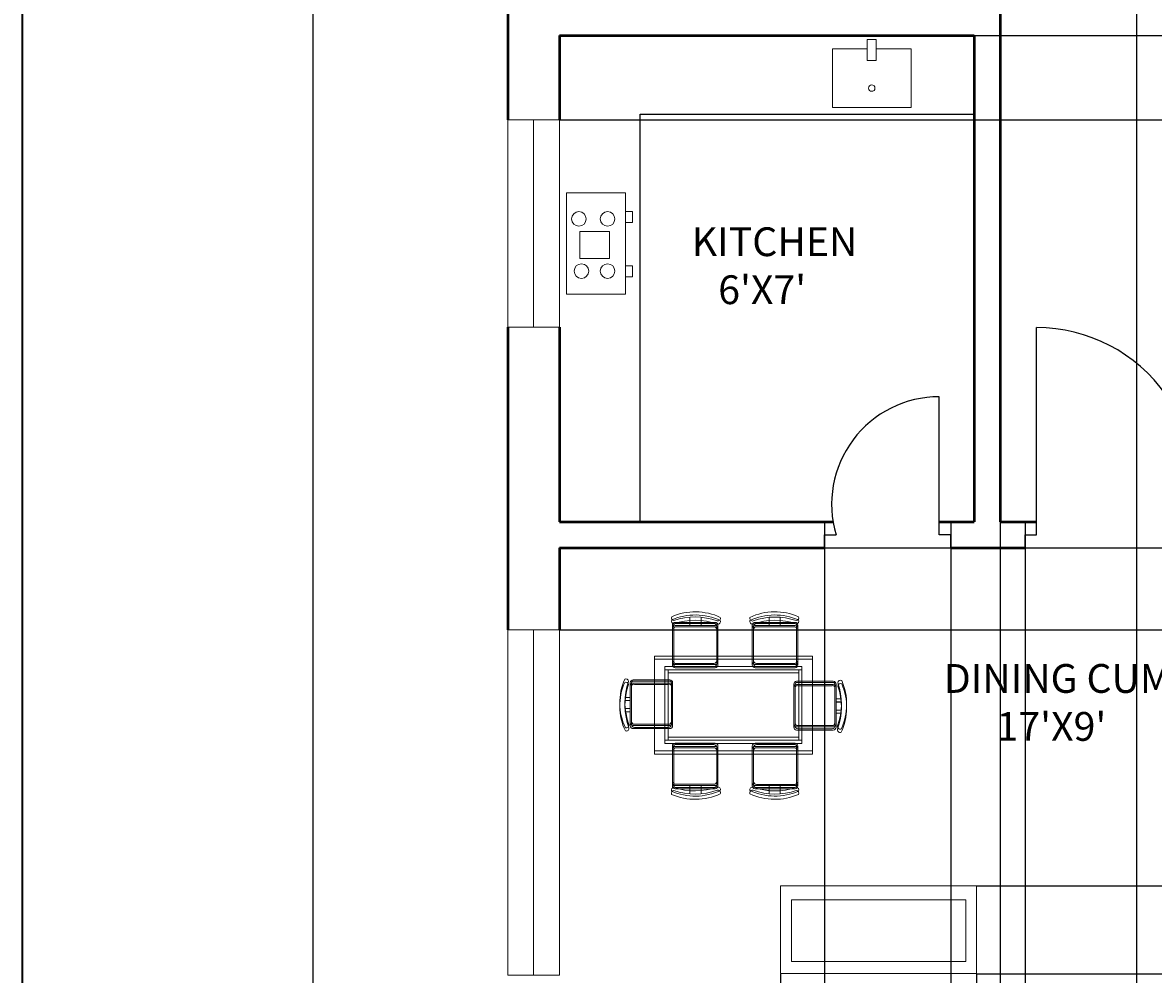
# Model space of a CAD drawing. Units: inches. Extents: x 2310 to 2937, y 1113 to 2410.
# Tile 17 of 23: x 2310 to 2507, y 2132 to 2297. Entities that reach past the tile are written whole.
import ezdxf

# ---------------------------------------------------------------- set-up
doc = ezdxf.new("R2010")
doc.units = ezdxf.units.IN
for name, color, linetype, lineweight in [('A-ANNO-DIMS', 2, 'Continuous', 18), ('A-ANNO-TTLB', 7, 'Continuous', 35), ('A-AREA-IDEN', 7, 'Continuous', 18), ('A-DOOR', 31, 'Continuous', 25), ('A-EQPM', 8, 'Continuous', 18), ('A-FLOR-CASE', 7, 'Continuous', 25), ('A-FLOR-FIXT', 9, 'Continuous', 18), ('A-FURN', 8, 'Continuous', 18), ('A-GLAZ', 191, 'Continuous', 20), ('A-WALL', 7, 'Continuous', 50)]:
    doc.layers.add(name, color=color, linetype=linetype, lineweight=lineweight)
doc.styles.get("Standard").update_dxf_attribs({"font": 'arial.ttf'})
doc.dimstyles.get("Standard").update_dxf_attribs({"dimtxt": 0.18, "dimasz": 0.18, "dimexe": 0.18, "dimexo": 0.0625, "dimgap": 0.09, "dimtad": 0, "dimtih": 1, "dimtoh": 1, "dimdec": 4, "dimzin": 0, "dimdsep": 46, "dimtxsty": 'Standard', "dimcen": 0.09, "dimadec": 0, "dimazin": 0, "dimtfac": 1, "dimtdec": 4, "dimtofl": 0, "dimtmove": 0, "dimatfit": 3, "dimfxl": 1, "dimtolj": 1, "dimtzin": 0, "dimarcsym": 0})

# ---------------------------------------------------------------- blocks, each defined once
blk = doc.blocks.new('SINK-KITCHEN')
blk.add_lwpolyline([(6.01, 11.79), (7.56, 11.79), (7.56, 8.11), (6.01, 8.11)], close=True)
blk.add_lwpolyline([(7.56, 10.17), (13.64, 10.17), (13.64, 0), (0, 0), (0, 10.17), (6.01, 10.17)])
blk.add_circle((6.79, 3.34), 0.556)
blk = doc.blocks.new('RANGE-4-BURNER')
for points in [[(1.2, 17.61), (1.2, 17.61), (1.2, 17.61), (1.2, 17.61)], [(1.2, 17.61), (11.5, 17.61), (11.5, 0), (1.2, 0)], [(1.2, 14.58), (0, 14.58), (0, 12.67), (1.2, 12.67)], [(4.01, 11.43), (9.13, 11.43), (9.13, 6.73), (4.01, 6.73)], [(1.2, 5.14), (0, 5.14), (0, 3.24), (1.2, 3.24)]]:
    blk.add_lwpolyline(points, close=True)
for centre in [(4.34, 13.6), (8.87, 13.6), (4.34, 4.53), (9.32, 4.53)]:
    blk.add_circle(centre, 1.27)
blk = doc.blocks.new('WIN-60IN')
for p, q in [((4.5, 60), (0, 60)), ((0, 60), (9, 60)), ((0, 60), (0, 0)), ((4.5, 0), (4.5, 60)), ((9, 60), (9, 0)), ((0, 0), (9, 0)), ((9, 0), (4.5, 0))]:
    blk.add_line(p, q)
blk = doc.blocks.new('DINING-TABLE')
for points in [[(0, 17.02), (27.45, 17.02), (27.45, 0.55), (0, 0.55)], [(0, 17.02), (27.45, 17.02), (27.45, 0.55), (0, 0.55)], [(0, 16.47), (27.45, 16.47), (27.45, 0), (0, 0)], [(0, 16.47), (27.45, 16.47), (27.45, 0), (0, 0)], [(1.83, 15.19), (25.62, 15.19), (25.62, 2.38), (1.83, 2.38)], [(1.83, 15.19), (25.62, 15.19), (25.62, 2.38), (1.83, 2.38)], [(1.83, 14.64), (25.62, 14.64), (25.62, 1.83), (1.83, 1.83)], [(1.83, 14.64), (25.62, 14.64), (25.62, 1.83), (1.83, 1.83)], [(2.38, 14.64), (25.07, 14.64), (25.07, 2.93), (2.38, 2.93)], [(2.38, 14.64), (25.07, 14.64), (25.07, 2.93), (2.38, 2.93)], [(2.38, 14.09), (25.07, 14.09), (25.07, 2.38), (2.38, 2.38)], [(2.38, 14.09), (25.07, 14.09), (25.07, 2.38), (2.38, 2.38)]]:
    blk.add_lwpolyline(points, close=True)
blk = doc.blocks.new('CHAIR-DINING')
for points in [[(0.62, 8.14, -0.578392), (0.05, 8.77, -0.214524), (8.49, 8.88, -0.552014), (8.09, 8.2, 0.175809), (0.62, 8.14)], [(0.62, 8.14, -0.578392), (0.05, 8.77, -0.214524), (8.49, 8.88, -0.552014), (8.09, 8.2, 0.175809), (0.62, 8.14)], [(0.62, 7.6, -0.578392), (0.05, 8.22, -0.214524), (8.49, 8.33, -0.552014), (8.09, 7.65, 0.175809), (0.62, 7.6)], [(0.62, 7.6, -0.578392), (0.05, 8.22, -0.214524), (8.49, 8.33, -0.552014), (8.09, 7.65, 0.175809), (0.62, 7.6)], [(7.88, 7.9, -0.414214), (8.36, 7.42), (8.36, 1.03, -0.414214), (7.88, 0.55), (0.94, 0.55, -0.414214), (0.45, 1.03), (0.45, 7.42, -0.414214), (0.94, 7.9), (7.88, 7.9)], [(7.88, 7.9, -0.414214), (8.36, 7.42), (8.36, 1.03, -0.414214), (7.88, 0.55), (0.94, 0.55, -0.414214), (0.45, 1.03), (0.45, 7.42, -0.414214), (0.94, 7.9), (7.88, 7.9)], [(3.37, 7.9), (3.37, 8.78, 0.064759)], [(3.37, 7.9), (3.37, 8.78, 0.064759)], [(3.37, 7.35), (3.37, 8.23, 0.064759)], [(3.37, 7.35), (3.37, 8.23, 0.064759)], [(7.88, 7.35, -0.414214), (8.36, 6.87), (8.36, 0.49, -0.414214), (7.88, 0), (0.94, 0, -0.414214), (0.45, 0.49), (0.45, 6.87, -0.414214), (0.94, 7.35), (7.88, 7.35)], [(7.88, 7.35, -0.414214), (8.36, 6.87), (8.36, 0.49, -0.414214), (7.88, 0), (0.94, 0, -0.414214), (0.45, 0.49), (0.45, 6.87, -0.414214), (0.94, 7.35), (7.88, 7.35)]]:
    blk.add_lwpolyline(points, format="xyb")
for points in [[(5.32, 8.8), (5.32, 7.9)], [(5.32, 8.79), (5.32, 7.9)], [(5.32, 8.25), (5.32, 7.35)], [(5.32, 8.25), (5.32, 7.35)]]:
    blk.add_lwpolyline(points)
for points in [[(7.87, 7.68), (1.16, 7.68, 0.414214), (0.67, 7.2), (0.67, 1.25, 0.414214), (1.16, 0.77), (7.87, 0.77, 0.512069), (8.14, 1.25), (8.14, 7.2, 0.512069)], [(7.87, 7.68), (1.16, 7.68, 0.414214), (0.67, 7.2), (0.67, 1.25, 0.414214), (1.16, 0.77), (7.87, 0.77, 0.512069), (8.14, 1.25), (8.14, 7.2, 0.512069)], [(7.87, 7.13), (1.16, 7.13, 0.414214), (0.67, 6.65), (0.67, 0.7, 0.414214), (1.16, 0.22), (7.87, 0.22, 0.512069), (8.14, 0.7), (8.14, 6.65, 0.512069)], [(7.87, 7.13), (1.16, 7.13, 0.414214), (0.67, 6.65), (0.67, 0.7, 0.414214), (1.16, 0.22), (7.87, 0.22, 0.512069), (8.14, 0.7), (8.14, 6.65, 0.512069)]]:
    blk.add_lwpolyline(points, format="xyb", close=True)
blk = doc.blocks.new('CHAIR-DINING-2')
for points in [[(7.63, 2.7), (0.69, 2.7, -0.414214), (0.2, 3.18), (0.2, 9.57, -0.414214), (0.69, 10.05), (7.63, 10.05, -0.414214), (8.11, 9.57), (8.11, 3.18, -0.414214), (7.63, 2.7)], [(7.63, 2.7), (0.69, 2.7, -0.414214), (0.2, 3.18), (0.2, 9.57, -0.414214), (0.69, 10.05), (7.63, 10.05, -0.414214), (8.11, 9.57), (8.11, 3.18, -0.414214), (7.63, 2.7)], [(7.63, 2.15), (0.69, 2.15, -0.414214), (0.2, 2.64), (0.2, 9.02, -0.414214), (0.69, 9.5), (7.63, 9.5, -0.414214), (8.11, 9.02), (8.11, 2.64, -0.414214), (7.63, 2.15)], [(7.63, 2.15), (0.69, 2.15, -0.414214), (0.2, 2.64), (0.2, 9.02, -0.414214), (0.69, 9.5), (7.63, 9.5, -0.414214), (8.11, 9.02), (8.11, 2.64, -0.414214), (7.63, 2.15)], [(7.95, 2.46, -0.578392), (8.51, 1.83, -0.214524), (0.07, 1.72, -0.552014), (0.47, 2.4, 0.175809), (7.95, 2.46)], [(7.95, 2.46, -0.578392), (8.51, 1.83, -0.214524), (0.07, 1.72, -0.552014), (0.47, 2.4, 0.175809), (7.95, 2.46)], [(5.19, 2.7), (5.19, 1.82, 0.064759)], [(5.19, 2.7), (5.19, 1.82, 0.064759)], [(5.19, 2.15), (5.19, 1.27, 0.064759)], [(5.19, 2.15), (5.19, 1.27, 0.064759)], [(7.95, 1.91, -0.578392), (8.51, 1.28, -0.214524), (0.07, 1.17, -0.552014), (0.47, 1.85, 0.175809), (7.95, 1.91)], [(7.95, 1.91, -0.578392), (8.51, 1.28, -0.214524), (0.07, 1.17, -0.552014), (0.47, 1.85, 0.175809), (7.95, 1.91)]]:
    blk.add_lwpolyline(points, format="xyb")
for points in [[(0.69, 2.92), (7.41, 2.92, 0.414214), (7.9, 3.4), (7.9, 9.35, 0.414214), (7.41, 9.83), (0.69, 9.83, 0.512069), (0.42, 9.35), (0.42, 3.4, 0.512069)], [(0.69, 2.92), (7.41, 2.92, 0.414214), (7.9, 3.4), (7.9, 9.35, 0.414214), (7.41, 9.83), (0.69, 9.83, 0.512069), (0.42, 9.35), (0.42, 3.4, 0.512069)], [(0.69, 2.37), (7.41, 2.37, 0.414214), (7.9, 2.85), (7.9, 8.8, 0.414214), (7.41, 9.28), (0.69, 9.28, 0.512069), (0.42, 8.8), (0.42, 2.85, 0.512069)], [(0.69, 2.37), (7.41, 2.37, 0.414214), (7.9, 2.85), (7.9, 8.8, 0.414214), (7.41, 9.28), (0.69, 9.28, 0.512069), (0.42, 8.8), (0.42, 2.85, 0.512069)]]:
    blk.add_lwpolyline(points, format="xyb", close=True)
for points in [[(3.25, 1.81), (3.25, 2.7)], [(3.25, 1.81), (3.25, 2.7)], [(3.25, 1.26), (3.25, 2.15)], [(3.25, 1.26), (3.25, 2.15)]]:
    blk.add_lwpolyline(points)
blk = doc.blocks.new('*D40')
at = {"layer": 'A-ANNO-DIMS', "color": 0, "lineweight": -2, "transparency": 16777216}
for p, q in [((2394.42, 2356.51), (2360.46, 2356.51)), ((2360.64, 2356.33), (2360.64, 2046.7)), ((2360.64, 1736.69), (2360.64, 2046.33)), ((2394.42, 1736.51), (2360.46, 1736.51))]:
    blk.add_line(p, q, dxfattribs=at)
at = {"layer": 'A-ANNO-DIMS', "color": 0, "transparency": 16777216}
for points in [[(2360.61, 2356.33), (2360.67, 2356.33), (2360.64, 2356.51)], [(2360.61, 1736.69), (2360.67, 1736.69), (2360.64, 1736.51)]]:
    blk.add_solid(points, dxfattribs=at)
at = {"layer": 'Defpoints', "color": 0, "transparency": 16777216}
for p in [(2360.64, 2356.51), (2394.49, 2356.51), (2394.49, 1736.51)]:
    blk.add_point(p, dxfattribs=at)
at = {"layer": 'A-ANNO-DIMS', "color": 0, "transparency": 16777216, "insert": (2360.64, 2046.51), "char_height": 0.18, "attachment_point": 5}
blk.add_mtext('\\A1;620', dxfattribs=at)
blk = doc.blocks.new('*D41')
at = {"layer": 'A-ANNO-DIMS', "color": 0, "lineweight": -2, "transparency": 16777216}
for p, q in [((2479.99, 2347.45), (2479.99, 1649.5)), ((2503.66, 2347.45), (2503.66, 1649.5)), ((2480.17, 1649.68), (2491.36, 1649.68)), ((2503.48, 1649.68), (2492.29, 1649.68))]:
    blk.add_line(p, q, dxfattribs=at)
at = {"layer": 'A-ANNO-DIMS', "color": 0, "transparency": 16777216}
for points in [[(2480.17, 1649.71), (2480.17, 1649.65), (2479.99, 1649.68)], [(2503.48, 1649.71), (2503.48, 1649.65), (2503.66, 1649.68)]]:
    blk.add_solid(points, dxfattribs=at)
at = {"layer": 'Defpoints', "color": 0, "transparency": 16777216}
for p in [(2479.99, 2347.51), (2503.66, 2347.51), (2503.66, 1649.68)]:
    blk.add_point(p, dxfattribs=at)
at = {"layer": 'A-ANNO-DIMS', "color": 0, "transparency": 16777216, "insert": (2491.82, 1649.68), "char_height": 0.18, "attachment_point": 5}
blk.add_mtext('\\A1;23.676', dxfattribs=at)
blk = doc.blocks.new('*D53')
at = {"layer": 'A-ANNO-DIMS', "color": 0, "lineweight": -2, "transparency": 16777216}
for p, q in [((2403.55, 2295.01), (2858.02, 2295.01)), ((2857.84, 2294.83), (2857.84, 2287.87)), ((2857.84, 2280.55), (2857.84, 2287.51)), ((2403.55, 2280.37), (2858.02, 2280.37))]:
    blk.add_line(p, q, dxfattribs=at)
at = {"layer": 'A-ANNO-DIMS', "color": 0, "transparency": 16777216}
for points in [[(2857.81, 2294.83), (2857.87, 2294.83), (2857.84, 2295.01)], [(2857.81, 2280.55), (2857.87, 2280.55), (2857.84, 2280.37)]]:
    blk.add_solid(points, dxfattribs=at)
at = {"layer": 'Defpoints', "color": 0, "transparency": 16777216}
for p in [(2403.49, 2295.01), (2403.49, 2280.37), (2857.84, 2280.37)]:
    blk.add_point(p, dxfattribs=at)
at = {"layer": 'A-ANNO-DIMS', "color": 0, "transparency": 16777216, "insert": (2857.84, 2287.69), "char_height": 0.18, "attachment_point": 5}
blk.add_mtext('\\A1;14.644', dxfattribs=at)
blk = doc.blocks.new('*D54')
at = {"layer": 'A-ANNO-DIMS', "color": 0, "lineweight": -2, "transparency": 16777216}
for p, q in [((2403.55, 2206.01), (2858.02, 2206.01)), ((2857.84, 2205.83), (2857.84, 2199.07)), ((2857.84, 2191.94), (2857.84, 2198.7)), ((2403.55, 2191.76), (2858.02, 2191.76))]:
    blk.add_line(p, q, dxfattribs=at)
at = {"layer": 'A-ANNO-DIMS', "color": 0, "transparency": 16777216}
for points in [[(2857.81, 2205.83), (2857.87, 2205.83), (2857.84, 2206.01)], [(2857.81, 2191.94), (2857.87, 2191.94), (2857.84, 2191.76)]]:
    blk.add_solid(points, dxfattribs=at)
at = {"layer": 'Defpoints', "color": 0, "transparency": 16777216}
for p in [(2403.49, 2206.01), (2403.49, 2191.76), (2857.84, 2191.76)]:
    blk.add_point(p, dxfattribs=at)
at = {"layer": 'A-ANNO-DIMS', "color": 0, "transparency": 16777216, "insert": (2857.84, 2198.89), "char_height": 0.18, "attachment_point": 5}
blk.add_mtext('\\A1;14.255', dxfattribs=at)
blk = doc.blocks.new('*D60')
at = {"layer": 'A-ANNO-DIMS', "color": 0, "lineweight": -2, "transparency": 16777216}
for p, q in [((2449.5, 2205.95), (2449.5, 1649.5)), ((2471.44, 2205.95), (2471.44, 1649.5)), ((2449.68, 1649.68), (2460.01, 1649.68)), ((2471.26, 1649.68), (2460.94, 1649.68))]:
    blk.add_line(p, q, dxfattribs=at)
at = {"layer": 'A-ANNO-DIMS', "color": 0, "transparency": 16777216}
for points in [[(2449.68, 1649.71), (2449.68, 1649.65), (2449.5, 1649.68)], [(2471.26, 1649.71), (2471.26, 1649.65), (2471.44, 1649.68)]]:
    blk.add_solid(points, dxfattribs=at)
at = {"layer": 'Defpoints', "color": 0, "transparency": 16777216}
for p in [(2449.5, 2206.01), (2471.44, 2206.01), (2471.44, 1649.68)]:
    blk.add_point(p, dxfattribs=at)
at = {"layer": 'A-ANNO-DIMS', "color": 0, "transparency": 16777216, "insert": (2460.47, 1649.68), "char_height": 0.18, "attachment_point": 5}
blk.add_mtext('\\A1;21.936', dxfattribs=at)
blk = doc.blocks.new('*D61')
at = {"layer": 'A-ANNO-DIMS', "color": 0, "lineweight": -2, "transparency": 16777216}
for p, q in [((2484.33, 2205.95), (2484.33, 1649.5)), ((2514.27, 2205.95), (2514.27, 1649.5)), ((2484.51, 1649.68), (2498.9, 1649.68)), ((2514.09, 1649.68), (2499.69, 1649.68))]:
    blk.add_line(p, q, dxfattribs=at)
at = {"layer": 'A-ANNO-DIMS', "color": 0, "transparency": 16777216}
for points in [[(2484.51, 1649.71), (2484.51, 1649.65), (2484.33, 1649.68)], [(2514.09, 1649.71), (2514.09, 1649.65), (2514.27, 1649.68)]]:
    blk.add_solid(points, dxfattribs=at)
at = {"layer": 'Defpoints', "color": 0, "transparency": 16777216}
for p in [(2484.33, 2206.01), (2514.27, 2206.01), (2514.27, 1649.68)]:
    blk.add_point(p, dxfattribs=at)
at = {"layer": 'A-ANNO-DIMS', "color": 0, "transparency": 16777216, "insert": (2499.3, 1649.68), "char_height": 0.18, "attachment_point": 5}
blk.add_mtext('\\A1;29.94', dxfattribs=at)
blk = doc.blocks.new('*D69')
at = {"layer": 'A-ANNO-DIMS', "color": 0, "lineweight": -2, "transparency": 16777216}
for p, q in [((2441.86, 2131.96), (2441.86, 1649.5)), ((2475.89, 2131.96), (2475.89, 1649.5)), ((2442.04, 1649.68), (2458.48, 1649.68)), ((2475.71, 1649.68), (2459.27, 1649.68))]:
    blk.add_line(p, q, dxfattribs=at)
at = {"layer": 'A-ANNO-DIMS', "color": 0, "transparency": 16777216}
for points in [[(2442.04, 1649.71), (2442.04, 1649.65), (2441.86, 1649.68)], [(2475.71, 1649.71), (2475.71, 1649.65), (2475.89, 1649.68)]]:
    blk.add_solid(points, dxfattribs=at)
at = {"layer": 'Defpoints', "color": 0, "transparency": 16777216}
for p in [(2441.86, 2132.02), (2475.89, 2132.02), (2475.89, 1649.68)]:
    blk.add_point(p, dxfattribs=at)
at = {"layer": 'A-ANNO-DIMS', "color": 0, "transparency": 16777216, "insert": (2458.88, 1649.68), "char_height": 0.18, "attachment_point": 5}
blk.add_mtext('\\A1;34.03', dxfattribs=at)
blk = doc.blocks.new('*D70')
at = {"layer": 'A-ANNO-DIMS', "color": 0, "lineweight": -2, "transparency": 16777216}
for p, q in [((2475.96, 2147.28), (2858.02, 2147.28)), ((2857.84, 2147.1), (2857.84, 2139.83)), ((2857.84, 2132.2), (2857.84, 2139.47)), ((2475.96, 2132.02), (2858.02, 2132.02))]:
    blk.add_line(p, q, dxfattribs=at)
at = {"layer": 'A-ANNO-DIMS', "color": 0, "transparency": 16777216}
for points in [[(2857.81, 2147.1), (2857.87, 2147.1), (2857.84, 2147.28)], [(2857.81, 2132.2), (2857.87, 2132.2), (2857.84, 2132.02)]]:
    blk.add_solid(points, dxfattribs=at)
at = {"layer": 'Defpoints', "color": 0, "transparency": 16777216}
for p in [(2475.89, 2147.28), (2857.84, 2147.28), (2475.89, 2132.02)]:
    blk.add_point(p, dxfattribs=at)
at = {"layer": 'A-ANNO-DIMS', "color": 0, "transparency": 16777216, "insert": (2857.84, 2139.65), "char_height": 0.18, "attachment_point": 5}
blk.add_mtext('\\A1;15.257', dxfattribs=at)

msp = doc.modelspace()

# ---------------------------------------------------------------- linework, layer by layer
at = {"layer": 'A-ANNO-TTLB'}
msp.add_lwpolyline([(2310.2498, 2409.8427), (2937.0534, 2409.8427), (2937.0534, 1616.036), (2310.2498, 1616.036)], close=True, dxfattribs=at)
at = {"layer": 'A-DOOR'}
for p, q in [((2486.3278, 2208.2639), (2486.3278, 2244.2639)), ((2469.4388, 2208.2639), (2469.4388, 2232.2639)), ((2449.5024, 2210.5139), (2449.5024, 2206.0139)), ((2471.4388, 2210.5139), (2471.4388, 2206.0139)), ((2484.3278, 2210.5139), (2484.3278, 2206.0139)), ((2449.5024, 2206.0139), (2449.5024, 2208.2639)), ((2449.5024, 2208.2639), (2451.5024, 2208.2639)), ((2471.4388, 2208.2639), (2469.4388, 2208.2639)), ((2471.4388, 2206.0139), (2471.4388, 2208.2639)), ((2484.3278, 2206.0139), (2484.3278, 2208.2639)), ((2484.3278, 2208.2639), (2486.3278, 2208.2639))]:
    msp.add_line(p, q, dxfattribs=at)
for centre, radius, start, end in [((2486.3278, 2216.7342), 27.5298, 340.442065, 90), ((2469.4388, 2213.5616), 18.7023, 90, 196.455037)]:
    msp.add_arc(centre, radius, start, end, dxfattribs=at)
at = {"layer": 'A-FLOR-CASE'}
for p, q in [((2417.517, 2210.5139), (2417.517, 2281.346)), ((2417.517, 2281.346), (2471.5691, 2281.346)), ((2471.5691, 2281.346), (2475.4859, 2281.346))]:
    msp.add_line(p, q, dxfattribs=at)
at = {"layer": 'A-FURN'}
for points in [[(2423.3618, 2193.3629, -0.17580919), (2430.8373, 2193.3063, 0.57839206), (2431.4036, 2193.929, 0.21452438), (2422.9654, 2194.0423, 0.55201397), (2423.3618, 2193.3629, -0.06507904)], [(2423.3618, 2193.3626, -0.17580919), (2430.8373, 2193.306, 0.57839206), (2431.4036, 2193.9287, 0.21452438), (2422.9654, 2194.042, 0.55201397), (2423.3618, 2193.3626, -0.06507904)], [(2423.3618, 2192.814, -0.17580919), (2430.8373, 2192.7574, 0.57839206), (2431.4036, 2193.3801, 0.21452438), (2422.9654, 2193.4933, 0.55201397), (2423.3618, 2192.814, -0.06507904)], [(2423.3618, 2192.8137, -0.17580919), (2430.8373, 2192.7571, 0.57839206), (2431.4036, 2193.3798, 0.21452438), (2422.9654, 2193.493, 0.55201397), (2423.3618, 2192.8137, -0.06507904)], [(2428.0825, 2193.0629), (2428.0825, 2193.9406, -0.06475861)], [(2428.0825, 2193.0626), (2428.0825, 2193.9403, -0.06475861)], [(2430.5201, 2193.0629), (2423.5802, 2193.0629, 0.41421356), (2423.0946, 2192.5774), (2423.0946, 2186.1962, 0.41421356), (2423.5802, 2185.7107), (2430.5201, 2185.7107, 0.41421356), (2431.0056, 2186.1962), (2431.0056, 2192.5774, 0.41421356), (2430.5201, 2193.0629)], [(2430.5201, 2192.514), (2423.5802, 2192.514, 0.41421356), (2423.0946, 2192.0285), (2423.0946, 2185.6473, 0.41421356), (2423.5802, 2185.1618), (2430.5201, 2185.1618, 0.41421356), (2431.0056, 2185.6473), (2431.0056, 2192.0285, 0.41421356), (2430.5201, 2192.514)], [(2430.5201, 2193.0626), (2423.5802, 2193.0626, 0.41421356), (2423.0947, 2192.5771), (2423.0947, 2186.1959, 0.41421356), (2423.5802, 2185.7104), (2430.5201, 2185.7104, 0.41421356), (2431.0056, 2186.1959), (2431.0056, 2192.5771, 0.41421356), (2430.5201, 2193.0626)], [(2430.5201, 2192.5137), (2423.5802, 2192.5137, 0.41421356), (2423.0947, 2192.0282), (2423.0947, 2185.647, 0.41421356), (2423.5802, 2185.1615), (2430.5201, 2185.1615, 0.41421356), (2431.0056, 2185.647), (2431.0056, 2192.0282, 0.41421356), (2430.5201, 2192.5137)], [(2428.0825, 2192.514), (2428.0825, 2193.3917, -0.06475861)], [(2428.0825, 2192.5137), (2428.0825, 2193.3914, -0.06475861)], [(2415.5411, 2175.3109, -0.57839206), (2414.9184, 2174.7446, -0.21452438), (2414.8051, 2183.1827, -0.55201397), (2415.4845, 2182.7863, 0.17580937), (2415.5411, 2175.3109)], [(2415.5411, 2175.3106, -0.57839206), (2414.9184, 2174.7443, -0.21452438), (2414.8052, 2183.1825, -0.55201397), (2415.4845, 2182.786, 0.17580937), (2415.5411, 2175.3106)], [(2415.5411, 2174.762, -0.57839206), (2414.9184, 2174.1956, -0.21452438), (2414.8051, 2182.6338, -0.55201397), (2415.4845, 2182.2374, 0.17580937), (2415.5411, 2174.762)], [(2415.5411, 2174.7617, -0.57839206), (2414.9184, 2174.1954, -0.21452438), (2414.8052, 2182.6335, -0.55201397), (2415.4845, 2182.2371, 0.17580937), (2415.5411, 2174.7617)], [(2415.7845, 2182.568, -0.41421356), (2416.27, 2183.0535), (2422.6512, 2183.0535, -0.41421356), (2423.1367, 2182.568), (2423.1367, 2175.628, -0.41421356), (2422.6512, 2175.1425), (2416.27, 2175.1425, -0.41421356), (2415.7845, 2175.628), (2415.7845, 2182.568)], [(2415.7845, 2182.5677, -0.41421356), (2416.27, 2183.0532), (2422.6512, 2183.0532, -0.41421356), (2423.1367, 2182.5677), (2423.1367, 2175.6277, -0.41421356), (2422.6512, 2175.1422), (2416.27, 2175.1422, -0.41421356), (2415.7845, 2175.6277), (2415.7845, 2182.5677)], [(2415.7845, 2182.0191, -0.41421356), (2416.27, 2182.5046), (2422.6512, 2182.5046, -0.41421356), (2423.1367, 2182.0191), (2423.1367, 2175.0791, -0.41421356), (2422.6512, 2174.5936), (2416.27, 2174.5936, -0.41421356), (2415.7845, 2175.0791), (2415.7845, 2182.0191)], [(2415.7845, 2182.0188, -0.41421356), (2416.27, 2182.5043), (2422.6512, 2182.5043, -0.41421356), (2423.1367, 2182.0188), (2423.1367, 2175.0788, -0.41421356), (2422.6512, 2174.5933), (2416.27, 2174.5933, -0.41421356), (2415.7845, 2175.0788), (2415.7845, 2182.0188)], [(2451.522, 2182.3303, 0.41421356), (2451.0364, 2182.8158), (2444.6553, 2182.8158, 0.41421356), (2444.1698, 2182.3303), (2444.1698, 2175.3904, 0.41421356), (2444.6553, 2174.9048), (2451.0364, 2174.9048, 0.41421356), (2451.522, 2175.3904), (2451.522, 2182.3303)], [(2451.522, 2182.33, 0.41421356), (2451.0364, 2182.8155), (2444.6553, 2182.8155, 0.41421356), (2444.1698, 2182.33), (2444.1698, 2175.3901, 0.41421356), (2444.6553, 2174.9045), (2451.0364, 2174.9045, 0.41421356), (2451.522, 2175.3901), (2451.522, 2182.33)], [(2451.522, 2181.7814, 0.41421356), (2451.0364, 2182.2669), (2444.6553, 2182.2669, 0.41421356), (2444.1698, 2181.7814), (2444.1698, 2174.8414, 0.41421356), (2444.6553, 2174.3559), (2451.0364, 2174.3559, 0.41421356), (2451.522, 2174.8414), (2451.522, 2181.7814)], [(2451.522, 2181.7811, 0.41421356), (2451.0364, 2182.2666), (2444.6553, 2182.2666, 0.41421356), (2444.1698, 2181.7811), (2444.1698, 2174.8411, 0.41421356), (2444.6553, 2174.3556), (2451.0364, 2174.3556, 0.41421356), (2451.522, 2174.8411), (2451.522, 2181.7811)], [(2451.822, 2182.5486, -0.17580919), (2451.7654, 2175.0732, 0.57839206), (2452.3881, 2174.5069, 0.21452438), (2452.5013, 2182.9451, 0.55201397), (2451.822, 2182.5486, -0.06507904)], [(2451.822, 2182.5483, -0.17580919), (2451.7654, 2175.0729, 0.57839206), (2452.3881, 2174.5066, 0.21452438), (2452.5013, 2182.9448, 0.55201397), (2451.822, 2182.5483, -0.06507904)], [(2451.822, 2181.9997, -0.17580919), (2451.7654, 2174.5243, 0.57839206), (2452.3881, 2173.958, 0.21452438), (2452.5013, 2182.3961, 0.55201397), (2451.822, 2181.9997, -0.06507904)], [(2451.822, 2181.9994, -0.17580919), (2451.7654, 2174.524, 0.57839206), (2452.3881, 2173.9577, 0.21452438), (2452.5013, 2182.3959, 0.55201397), (2451.822, 2181.9994, -0.06507904)], [(2415.7845, 2178.0657), (2414.9068, 2178.0657, 0.06475861)], [(2415.7845, 2178.0654), (2414.9068, 2178.0654, 0.06475861)], [(2451.522, 2177.828), (2452.3996, 2177.828, -0.06475861)], [(2451.522, 2177.8277), (2452.3997, 2177.8277, -0.06475861)], [(2415.7845, 2177.5168), (2414.9068, 2177.5168, 0.06475861)], [(2415.7845, 2177.5165), (2414.9068, 2177.5165, 0.06475861)], [(2451.522, 2177.2791), (2452.3996, 2177.2791, -0.06475861)], [(2451.522, 2177.2788), (2452.3997, 2177.2788, -0.06475861)], [(2444.3877, 2164.6971, 0.41421356), (2444.8732, 2165.1827), (2444.8732, 2171.5638, 0.41421356), (2444.3877, 2172.0493), (2437.4478, 2172.0493, 0.41421356), (2436.9622, 2171.5638), (2436.9622, 2165.1827, 0.41421356), (2437.4478, 2164.6971), (2444.3877, 2164.6971)], [(2444.3877, 2164.6969, 0.41421356), (2444.8732, 2165.1824), (2444.8732, 2171.5635, 0.41421356), (2444.3877, 2172.0491), (2437.4478, 2172.0491, 0.41421356), (2436.9623, 2171.5635), (2436.9623, 2165.1824, 0.41421356), (2437.4478, 2164.6969), (2444.3877, 2164.6969)], [(2444.3877, 2164.1482, 0.41421356), (2444.8732, 2164.6338), (2444.8732, 2171.0149, 0.41421356), (2444.3877, 2171.5004), (2437.4478, 2171.5004, 0.41421356), (2436.9622, 2171.0149), (2436.9622, 2164.6338, 0.41421356), (2437.4478, 2164.1482), (2444.3877, 2164.1482)], [(2444.3877, 2164.1479, 0.41421356), (2444.8732, 2164.6335), (2444.8732, 2171.0146, 0.41421356), (2444.3877, 2171.5001), (2437.4478, 2171.5001, 0.41421356), (2436.9623, 2171.0146), (2436.9623, 2164.6335, 0.41421356), (2437.4478, 2164.1479), (2444.3877, 2164.1479)], [(2444.606, 2164.3971, -0.17580928), (2437.1306, 2164.4537, 0.57839206), (2436.5643, 2163.831, 0.21452438), (2445.0025, 2163.7178, 0.55201397), (2444.6061, 2164.3971, -0.06507904)], [(2444.6061, 2164.3968, -0.17580928), (2437.1306, 2164.4534, 0.57839206), (2436.5643, 2163.8307, 0.21452438), (2445.0025, 2163.7175, 0.55201397), (2444.6061, 2164.3968, -0.06507904)], [(2439.8854, 2164.6971), (2439.8854, 2163.8195, -0.06475861)], [(2439.8854, 2164.6969), (2439.8854, 2163.8192, -0.06475861)], [(2439.8854, 2164.1482), (2439.8854, 2163.2705, -0.06475861)], [(2439.8854, 2164.1479), (2439.8854, 2163.2703, -0.06475861)], [(2444.606, 2163.8482, -0.17580928), (2437.1306, 2163.9048, 0.57839206), (2436.5643, 2163.2821, 0.21452438), (2445.0025, 2163.1689, 0.55201397), (2444.6061, 2163.8482, -0.06507904)], [(2444.6061, 2163.8479, -0.17580928), (2437.1306, 2163.9045, 0.57839206), (2436.5643, 2163.2818, 0.21452438), (2445.0025, 2163.1686, 0.55201397), (2444.6061, 2163.8479, -0.06507904)]]:
    msp.add_lwpolyline(points, format="xyb", dxfattribs=at)
for points in [[(2426.1399, 2193.9565), (2426.1399, 2193.0629)], [(2426.1399, 2193.9562), (2426.1399, 2193.0626)], [(2426.1399, 2193.4076), (2426.1399, 2192.514)], [(2426.1399, 2193.4073), (2426.1399, 2192.5137)], [(2414.8909, 2180.0083), (2415.7845, 2180.0083)], [(2414.8909, 2180.008), (2415.7845, 2180.008)], [(2452.4156, 2179.7706), (2451.522, 2179.7706)], [(2452.4156, 2179.7703), (2451.522, 2179.7703)], [(2414.8909, 2179.4594), (2415.7845, 2179.4594)], [(2414.8909, 2179.4591), (2415.7845, 2179.4591)], [(2452.4156, 2179.2217), (2451.522, 2179.2217)], [(2452.4156, 2179.2214), (2451.522, 2179.2214)], [(2441.828, 2163.8035), (2441.828, 2164.6971)], [(2441.828, 2163.8032), (2441.828, 2164.6969)], [(2441.828, 2163.2546), (2441.828, 2164.1482)], [(2441.828, 2163.2543), (2441.828, 2164.1479)]]:
    msp.add_lwpolyline(points, dxfattribs=at)
for points in [[(2423.5831, 2192.8442), (2430.3014, 2192.8442, -0.41421356), (2430.7869, 2192.3586), (2430.7869, 2186.415, -0.41421356), (2430.3014, 2185.9294), (2423.5831, 2185.9294, -0.51206948), (2423.3134, 2186.415), (2423.3134, 2192.3586, -0.51206948)], [(2423.5831, 2192.8439), (2430.3014, 2192.8439, -0.41421356), (2430.7869, 2192.3583), (2430.7869, 2186.4147, -0.41421356), (2430.3014, 2185.9291), (2423.5831, 2185.9291, -0.51206948), (2423.3134, 2186.4147), (2423.3134, 2192.3583, -0.51206948)], [(2423.5831, 2192.2952), (2430.3014, 2192.2952, -0.41421356), (2430.7869, 2191.8097), (2430.7869, 2185.866, -0.41421356), (2430.3014, 2185.3805), (2423.5831, 2185.3805, -0.51206948), (2423.3134, 2185.866), (2423.3134, 2191.8097, -0.51206948)], [(2423.5831, 2192.295), (2430.3014, 2192.295, -0.41421356), (2430.7869, 2191.8094), (2430.7869, 2185.8658, -0.41421356), (2430.3014, 2185.3802), (2423.5831, 2185.3802, -0.51206948), (2423.3134, 2185.8658), (2423.3134, 2191.8094, -0.51206948)], [(2416.0032, 2182.565), (2416.0032, 2175.8468, 0.41421356), (2416.4888, 2175.3612), (2422.4324, 2175.3612, 0.41421356), (2422.918, 2175.8468), (2422.918, 2182.565, 0.51206948), (2422.4324, 2182.8348), (2416.4888, 2182.8348, 0.51206948)], [(2416.0032, 2182.5647), (2416.0032, 2175.8465, 0.41421356), (2416.4888, 2175.3609), (2422.4325, 2175.3609, 0.41421356), (2422.918, 2175.8465), (2422.918, 2182.5647, 0.51206948), (2422.4325, 2182.8345), (2416.4888, 2182.8345, 0.51206948)], [(2416.0032, 2182.0161), (2416.0032, 2175.2978, 0.41421356), (2416.4888, 2174.8123), (2422.4324, 2174.8123, 0.41421356), (2422.918, 2175.2978), (2422.918, 2182.0161, 0.51206948), (2422.4324, 2182.2859), (2416.4888, 2182.2859, 0.51206948)], [(2416.0032, 2182.0158), (2416.0032, 2175.2976, 0.41421356), (2416.4888, 2174.812), (2422.4325, 2174.812, 0.41421356), (2422.918, 2175.2976), (2422.918, 2182.0158, 0.51206948), (2422.4325, 2182.2856), (2416.4888, 2182.2856, 0.51206948)], [(2451.3032, 2182.3274), (2451.3032, 2175.6091, -0.41421356), (2450.8177, 2175.1236), (2444.874, 2175.1236, -0.41421356), (2444.3885, 2175.6091), (2444.3885, 2182.3274, -0.51206948), (2444.874, 2182.5971), (2450.8177, 2182.5971, -0.51206948)], [(2451.3032, 2182.3271), (2451.3032, 2175.6088, -0.41421356), (2450.8177, 2175.1233), (2444.874, 2175.1233, -0.41421356), (2444.3885, 2175.6088), (2444.3885, 2182.3271, -0.51206948), (2444.874, 2182.5968), (2450.8177, 2182.5968, -0.51206948)], [(2451.3032, 2181.7784), (2451.3032, 2175.0602, -0.41421356), (2450.8177, 2174.5746), (2444.874, 2174.5746, -0.41421356), (2444.3885, 2175.0602), (2444.3885, 2181.7784, -0.51206948), (2444.874, 2182.0482), (2450.8177, 2182.0482, -0.51206948)], [(2451.3032, 2181.7781), (2451.3032, 2175.0599, -0.41421356), (2450.8177, 2174.5744), (2444.874, 2174.5744, -0.41421356), (2444.3885, 2175.0599), (2444.3885, 2181.7781, -0.51206948), (2444.874, 2182.0479), (2450.8177, 2182.0479, -0.51206948)], [(2444.3848, 2164.9159), (2437.6665, 2164.9159, -0.41421356), (2437.181, 2165.4014), (2437.181, 2171.3451, -0.41421356), (2437.6665, 2171.8306), (2444.3848, 2171.8306, -0.51206948), (2444.6545, 2171.3451), (2444.6545, 2165.4014, -0.51206948)], [(2444.3848, 2164.9156), (2437.6665, 2164.9156, -0.41421356), (2437.181, 2165.4011), (2437.181, 2171.3448, -0.41421356), (2437.6665, 2171.8303), (2444.3848, 2171.8303, -0.51206948), (2444.6545, 2171.3448), (2444.6545, 2165.4011, -0.51206948)], [(2444.3848, 2164.367), (2437.6665, 2164.367, -0.41421356), (2437.181, 2164.8525), (2437.181, 2170.7962, -0.41421356), (2437.6665, 2171.2817), (2444.3848, 2171.2817, -0.51206948), (2444.6545, 2170.7962), (2444.6545, 2164.8525, -0.51206948)], [(2444.3848, 2164.3667), (2437.6665, 2164.3667, -0.41421356), (2437.181, 2164.8522), (2437.181, 2170.7959, -0.41421356), (2437.6665, 2171.2814), (2444.3848, 2171.2814, -0.51206948), (2444.6545, 2170.7959), (2444.6545, 2164.8522, -0.51206948)]]:
    msp.add_lwpolyline(points, format="xyb", close=True, dxfattribs=at)
for points in [[(2441.8613, 2147.2815), (2475.8929, 2147.2815), (2475.8929, 2132.0241), (2441.8613, 2132.0241)], [(2443.7686, 2144.837), (2474.0742, 2144.837), (2474.0742, 2134.1554), (2443.7686, 2134.1554)]]:
    msp.add_lwpolyline(points, close=True, dxfattribs=at)
at = {"layer": 'A-GLAZ'}
for p, q in [((2403.4859, 2280.3697), (2394.4859, 2280.3697)), ((2394.4859, 2280.3697), (2398.9859, 2280.3697)), ((2394.4859, 2280.3697), (2394.4859, 2244.3697)), ((2398.9859, 2280.3697), (2398.9859, 2244.3697)), ((2403.4859, 2280.3697), (2403.4859, 2244.3697)), ((2398.9859, 2244.3697), (2394.4859, 2244.3697)), ((2394.4859, 2244.3697), (2403.4859, 2244.3697))]:
    msp.add_line(p, q, dxfattribs=at)
at = {"layer": 'A-WALL'}
for p, q in [((2479.9859, 2321.7598), (2479.9859, 2210.5139)), ((2394.4859, 2313.9231), (2394.4859, 2280.3697)), ((2403.4859, 2295.0139), (2475.4859, 2295.0139)), ((2403.4859, 2295.0139), (2403.4859, 2280.3697)), ((2475.4859, 2295.0139), (2475.4859, 2210.5139)), ((2394.4859, 2244.3697), (2394.4859, 2191.7587)), ((2403.4859, 2244.3697), (2403.4859, 2210.5139)), ((2403.4859, 2210.5139), (2450.9864, 2210.5139)), ((2469.4388, 2210.5139), (2475.4859, 2210.5139)), ((2479.9859, 2210.5139), (2486.3278, 2210.5139)), ((2403.4859, 2206.0139), (2449.5024, 2206.0139)), ((2403.4859, 2206.0139), (2403.4859, 2191.7587)), ((2471.4388, 2206.0139), (2484.3278, 2206.0139))]:
    msp.add_line(p, q, dxfattribs=at)

# ---------------------------------------------------------------- block references
at = {"layer": 'A-EQPM', "rotation": 180}
msp.add_blockref('RANGE-4-BURNER', (2416.174, 2267.6901), dxfattribs=at)
at = {"layer": 'A-FLOR-FIXT'}
msp.add_blockref('SINK-KITCHEN', (2450.9184, 2282.5424), dxfattribs=at)
at = {"layer": 'A-FURN'}
for name, p in [('CHAIR-DINING', (2436.5112, 2185.1615)), ('DINING-TABLE', (2419.9671, 2170.1853)), ('CHAIR-DINING-2', (2422.8916, 2161.9978))]:
    msp.add_blockref(name, p, dxfattribs=at)
at = {"layer": 'A-GLAZ', "extrusion": (0, 0, -1), "zscale": -1}
msp.add_blockref('WIN-60IN', (-2403.4859, 2131.7587), dxfattribs=at)

# ---------------------------------------------------------------- texts
at = {"layer": 'A-AREA-IDEN', "char_height": 5, "attachment_point": 1}
for s, width, insert in [("    KITCHEN\\P       6'X7'", 139.317104, (2420.3493, 2261.69)), ("    DINING CUM LIVING\\P          17'X9'", 158.341629, (2464.1081, 2185.8129))]:
    msp.add_mtext_dynamic_manual_height_columns(s, width=width, gutter_width=12.5, heights=[0], dxfattribs=dict(at, insert=insert))

# ---------------------------------------------------------------- dimensions: what is measured, and where the dimension line sits
at = {"layer": 'A-ANNO-DIMS'}
for base, p1, p2, override, picture, middle in [((2360.6359, 2356.5139), (2394.4859, 1736.5139), (2394.4859, 2356.5139), {"dimdec": 0, "dimlfac": 1, "dimrnd": 0, "dimzin": 0, "dimdsep": 46, "dimlunit": 2}, '*D40', (2360.6359, 2046.5139)), ((2857.8359, 2280.3697), (2403.4859, 2295.0139), (2403.4859, 2280.3697), {"dimdec": 3, "dimlfac": 1, "dimrnd": 0, "dimzin": 0, "dimdsep": 46, "dimlunit": 2}, '*D53', (2857.8359, 2287.6918)), ((2857.8359, 2191.7587), (2403.4859, 2206.0139), (2403.4859, 2191.7587), {"dimdec": 3, "dimlfac": 1, "dimrnd": 0, "dimzin": 0, "dimdsep": 46, "dimlunit": 2}, '*D54', (2857.8359, 2198.8863)), ((2857.8359, 2147.2815), (2475.8929, 2132.0241), (2475.8929, 2147.2815), {"dimdec": 3, "dimlfac": 1, "dimrnd": 0, "dimzin": 0, "dimdsep": 46, "dimlunit": 2}, '*D70', (2857.8359, 2139.6528))]:
    dim = msp.add_linear_dim(base=base, p1=p1, p2=p2, angle=90, dimstyle='Standard', override=override, dxfattribs=at)
    dim.commit()
    dim.dimension.update_dxf_attribs({"geometry": picture, "text_midpoint": middle})
for base, p1, p2, override, picture, middle in [((2503.662, 1649.6807), (2479.9859, 2347.5139), (2503.662, 2347.5139), {"dimdec": 3, "dimlfac": 1, "dimrnd": 0, "dimzin": 0, "dimdsep": 46, "dimlunit": 2}, '*D41', (2491.824, 1649.6807)), ((2471.4388, 1649.6807), (2449.5024, 2206.0139), (2471.4388, 2206.0139), {"dimdec": 3, "dimlfac": 1, "dimrnd": 0, "dimzin": 0, "dimdsep": 46, "dimlunit": 2}, '*D60', (2460.4706, 1649.6807)), ((2514.2692, 1649.6807), (2484.3278, 2206.0139), (2514.2692, 2206.0139), {"dimdec": 2, "dimlfac": 1, "dimrnd": 0, "dimzin": 0, "dimdsep": 46, "dimlunit": 2}, '*D61', (2499.2985, 1649.6807)), ((2475.8929, 1649.6807), (2441.8613, 2132.0241), (2475.8929, 2132.0241), {"dimdec": 2, "dimlfac": 1, "dimrnd": 0, "dimzin": 0, "dimdsep": 46, "dimlunit": 2}, '*D69', (2458.8771, 1649.6807))]:
    dim = msp.add_linear_dim(base=base, p1=p1, p2=p2, dimstyle='Standard', override=override, dxfattribs=at)
    dim.commit()
    dim.dimension.update_dxf_attribs({"geometry": picture, "text_midpoint": middle})

doc.saveas('drawing.dxf')
